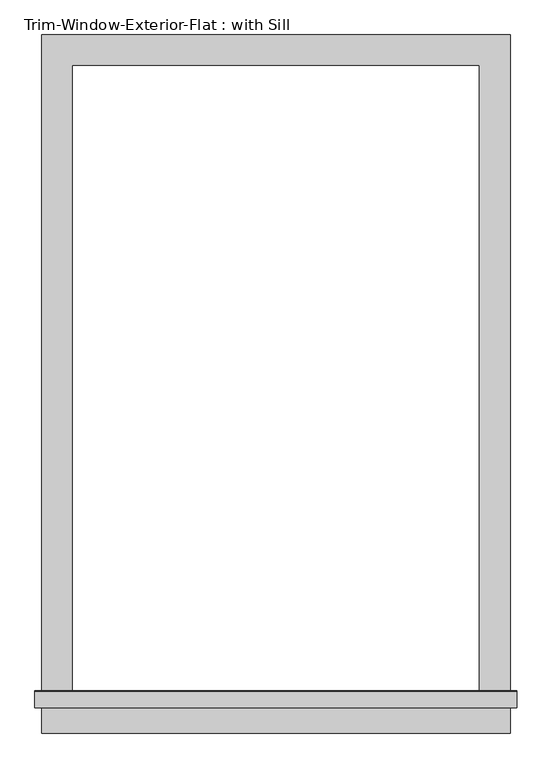
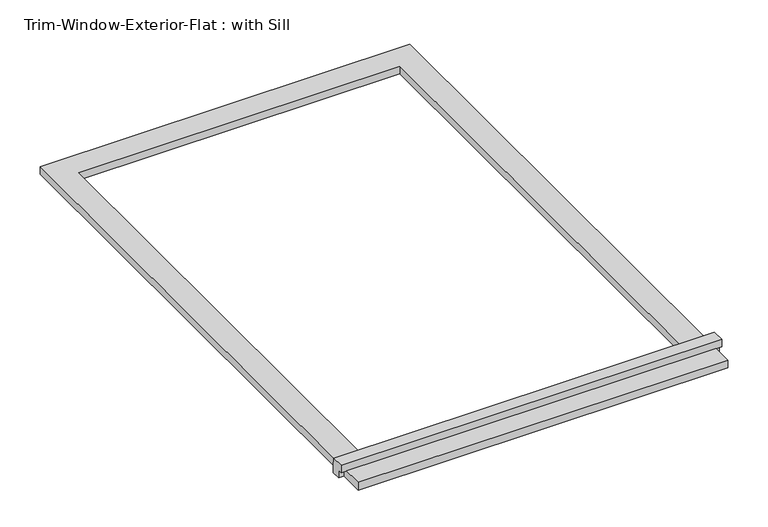
"""IFC4 building model written with IfcOpenShell, lengths in millimetres: proxy geometry, Trim-Window-Exterior-Flat : with Sill."""

from ifc_helpers import new_model, si_unit, frame, origin, origin_with_axes, place, context, project, spatial, polyline, outline, extrude, source, transform, mapped, element, save


def trim_window_exterior_flat_with_sill_6cd3ad68(model_context):
    return source(origin(), model_context, "Body", "SweptSolid", [
        extrude(outline(polyline([(438.15, -1190.5823709), (438.15, -1247.7323709), (-438.15, -1247.7323709), (-438.15, -1190.5823709), (438.15, -1190.5823709)])), origin_with_axes(), (0.0, 0.0, 1.0), 19.05),
        extrude(outline(polyline([(-1200.15, 38.1), (-1170.8580645, 38.1), (-1168.4, 19.05), (-1168.4, 0.0), (-1190.5823709, 0.0), (-1190.5823709, 19.05), (-1200.15, 19.05), (-1200.15, 38.1)])), frame((-450.85, 0.0, 0.0), z_axis=(1.0, 0.0, 0.0), x_axis=(0.0, 1.0, 0.0)), (0.0, 0.0, 1.0), 901.7),
        extrude(outline(polyline([(-438.15, 57.15), (438.15, 57.15), (438.15, -1168.4), (381.0, -1168.4), (381.0, 0.0), (-381.0, 0.0), (-381.0, -1168.4), (-438.15, -1168.4), (-438.15, 57.15)])), origin_with_axes(), (0.0, 0.0, 1.0), 19.05),
    ])


if __name__ == "__main__":
    model = new_model("IFC4")
    model_context = context("Model", 3, world=origin())
    ifc_project = project(units=[si_unit("LENGTHUNIT", "METRE", prefix="MILLI")], contexts=[model_context])
    site = spatial("IfcSite", under=ifc_project)
    building = spatial("IfcBuilding", under=site)
    placement = place(None, origin())
    trim_window_exterior_flat_with_sill_shape = trim_window_exterior_flat_with_sill_6cd3ad68(model_context)
    element("IfcBuildingElementProxy", 1, Name="Trim-Window-Exterior-Flat : with Sill", ObjectType="Trim-Window-Exterior-Flat : with Sill", at=placement, inside=building, context=model_context, shape_type="MappedRepresentation", body=[
        mapped(trim_window_exterior_flat_with_sill_shape, transform((0.0, 0.0, 0.0), x_axis=(1.0, 0.0, 0.0), y_axis=(0.0, 1.0, 0.0), z_axis=(0.0, 0.0, 1.0))),
    ])
    save(model, "model.ifc")

# Revit data of these elements
# Type "Trim-Window-Exterior-Flat : with Sill"
#   Trim Width = 0' - 2 1/4"
#   Trim Thickness_Picture Frame = 0' - 1 1/4"
#   Trim Thickness_with Sill = 0' - 0 3/4"
#   Sill Thickness = 0' - 1 1/4"
#   Opening Width [instance default] = 2' - 0"
#   Opening Height [instance default] = 3' - 0"
#   Default Elevation = 4' - 0"
#   Sill = yes
#   Picture Frame = no
#   Trim Material [instance default] = none
# Element 1 (IfcBuildingElementProxy, "Trim-Window-Exterior-Flat : with Sill")
#   Opening Width = 2' - 6"
#   Opening Height = 3' - 10"
#   Trim Material = Clad - White
#   Materials on its faces: "Clad - White"
# Materials
#   "Clad - White": class "Wood", colour RGB 242 242 238, transparency 0, Cost = 0
